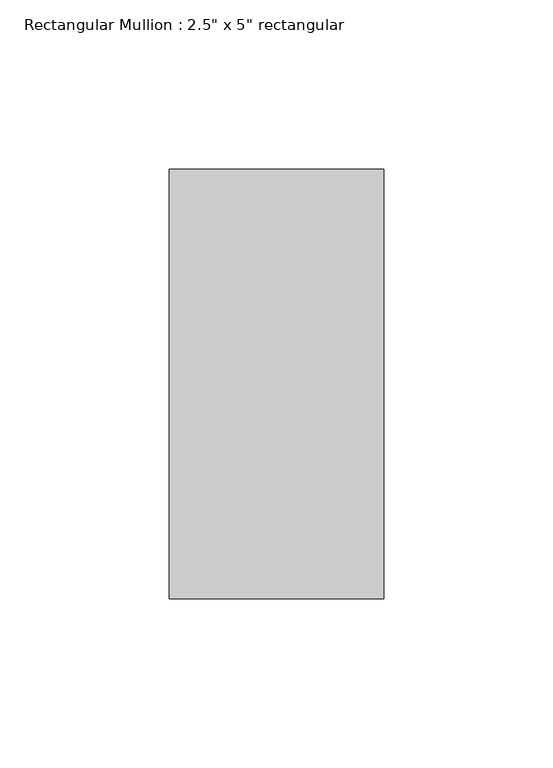
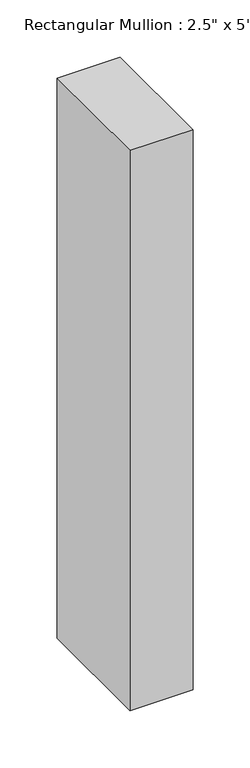
"""IFC4 building model written with IfcOpenShell, lengths in millimetres: member geometry."""

from ifc_helpers import new_model, si_unit, frame, origin, place, context, project, spatial, polyline, outline, extrude, source, transform, mapped, element, save


def member_a400357f(model_context):
    return source(origin(), model_context, "Body", "SweptSolid", [
        extrude(outline(polyline([(0.0, 63.5), (0.0, -63.5), (-63.5, -63.5), (-63.5, 63.5), (0.0, 63.5)])), frame((0.0, 0.0, -596.9), z_axis=(0.0, 0.0, 1.0), x_axis=(1.0, 0.0, 0.0)), (0.0, 0.0, 1.0), 596.9),
    ])


if __name__ == "__main__":
    model = new_model("IFC4")
    model_context = context("Model", 3, world=origin())
    ifc_project = project(units=[si_unit("LENGTHUNIT", "METRE", prefix="MILLI")], contexts=[model_context])
    site = spatial("IfcSite", under=ifc_project)
    building = spatial("IfcBuilding", under=site)
    placement = place(None, origin())
    member_shape = member_a400357f(model_context)
    element("IfcMember", 1, ObjectType="Rectangular Mullion : 2.5\" x 5\" rectangular", at=placement, inside=building, context=model_context, shape_type="MappedRepresentation", body=[
        mapped(member_shape, transform((0.0, 0.0, 0.0), x_axis=(1.0, 0.0, 0.0), y_axis=(0.0, 1.0, 0.0), z_axis=(0.0, 0.0, 1.0))),
    ])
    save(model, "model.ifc")

# Revit data of these elements
# Type "Rectangular Mullion : 2.5\" x 5\" rectangular"
#   built-in parameter 1007304 = 0.416667 (stored number, unit not read)
#   built-in parameter 1007301 = 0.104167 (stored number, unit not read)
#   built-in parameter 1007300 = 0.104167 (stored number, unit not read)
# Element 1 (IfcMember, "Rectangular Mullion : 2.5\" x 5\" rectangular")
#   Materials on its faces: "Aluminum"
# Materials
#   "Aluminum": class "Metal", colour RGB 247 247 247, transparency 0, Description = "Aluminum 6061", Cost = 0
